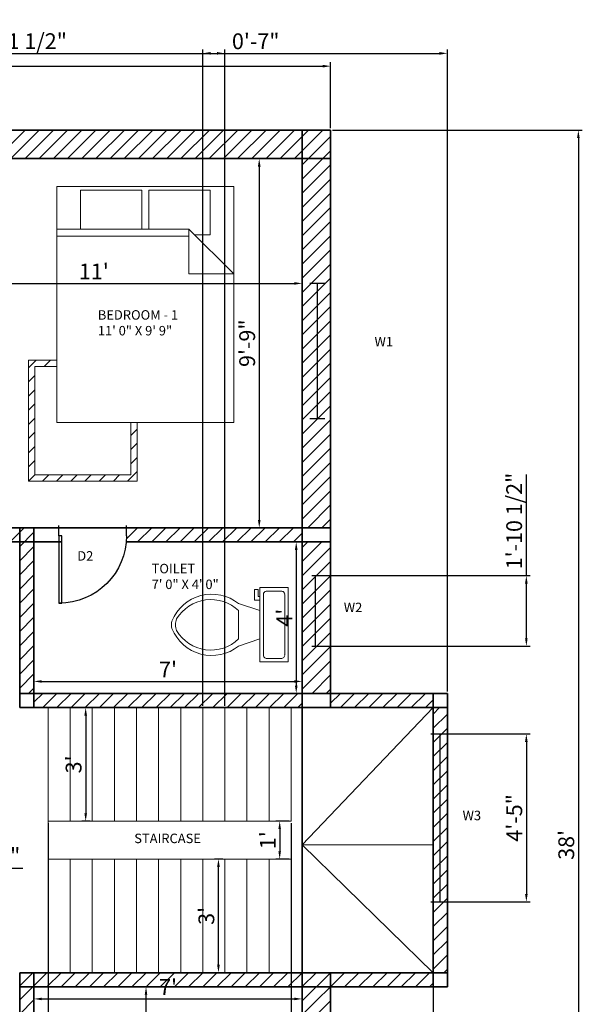
# Model space of a CAD drawing. Units: millimetres. Extents: x 2682 to 3042, y 1647 to 2164.
# Tile 4 of 4: x 2864 to 3042, y 1852 to 2164. Entities that reach past the tile are written whole.
import ezdxf

# ---------------------------------------------------------------- set-up
doc = ezdxf.new("R2010")
doc.units = ezdxf.units.MM
for name, color, linetype, lineweight in [('A-ANNO-TEXT', 170, 'Continuous', 18), ('A-AREA-IDEN', 170, 'Continuous', 18), ('A-FLOR-FIXT', 220, 'Continuous', 18), ('A-WALL-PATT', 3, 'Continuous', 13), ('dimensions', 140, 'Continuous', 18), ('doors', 40, 'Continuous', 25), ('furniture', 220, 'Continuous', 18), ('staircase', 10, 'Continuous', 18), ('walls', 70, 'Continuous', 35), ('windows', 50, 'Continuous', 25)]:
    doc.layers.add(name, color=color, linetype=linetype, lineweight=lineweight)
doc.layers.add('A-FURN-PATT', color=251, linetype='Continuous', lineweight=13, true_color=0x636466)
doc.styles.get("Standard").update_dxf_attribs({"font": 'arial.ttf'})
doc.dimstyles.new('ISO-25', dxfattribs={"dimtxt": 5, "dimasz": 2.5, "dimexe": 1.25, "dimexo": 0.625, "dimtad": 1, "dimdec": 0, "dimlunit": 3, "dimtxsty": 'Standard', "dimcen": 2.5, "dimadec": 0, "dimazin": 0, "dimtfac": 1, "dimtdec": 0, "dimtmove": 0, "dimatfit": 3, "dimfxl": 1, "dimarcsym": 0})

# ---------------------------------------------------------------- blocks, each defined once
blk = doc.blocks.new('*U2')
for p, q in [((0, 0), (0, -6)), ((40, 0), (40, -6))]:
    blk.add_line(p, q)
blk.add_lwpolyline([(0, 0), (0, 40), (1.75, 40), (1.75, 0)], close=True)
blk.add_arc((0, 0), 40, 0, 90)
blk = doc.blocks.new('*U4')
for p, q in [((0, 4), (0, 0)), ((36, 4), (36, 0)), ((0, 2), (36, 2))]:
    blk.add_line(p, q)
blk = doc.blocks.new('*U5')
for p, q in [((0, 4), (0, 0)), ((0, 2), (36, 2)), ((36, 4), (36, 0))]:
    blk.add_line(p, q)
blk = doc.blocks.new('*U6')
for p, q in [((0, 4), (0, 0)), ((36, 4), (36, 0)), ((0, 2), (36, 2))]:
    blk.add_line(p, q)
blk = doc.blocks.new('Toilet - top')
for p, q in [((9.5, -6), (9.5, -2)), ((-8, -8.5), (-8, -8)), ((-7, -8), (-7, -9.5)), ((-4, -8), (-6, -14)), ((4, -8), (6, -14)), ((-10, -8.5), (-8, -8.5)), ((-10, -9.5), (-10, -8.5)), ((-7, -9.5), (-10, -9.5)), ((4, -14), (-4, -14))]:
    blk.add_line(p, q)
blk.add_lwpolyline([(10.5, -8), (10.5, 0), (-10.5, 0), (-10.5, -8)], close=True)
for points in [[(-9.5, -2), (-9.5, -6)], [(8.5, -1), (-8.5, -1)], [(-8.5, -7), (8.5, -7)]]:
    blk.add_lwpolyline(points)
for centre, radius, start, end in [((-8.62, -1.88), 0.884, 81.8699, 188.1301), ((8.62, -1.88), 0.884, 351.8699, 98.1301), ((-8.62, -6.12), 0.884, 171.8699, 278.1301), ((8.62, -6.12), 0.884, 261.8699, 8.1301), ((3.52, -21.58), 12.17, 141.4691, 247.9714), ((4.2, -21.82), 11.33, 136.3677, 238.9468), ((-3.52, -21.58), 12.17, 292.0284, 38.5307), ((-4.2, -21.82), 11.33, 301.053, 43.6321), ((0, -27.88), 4, 245.7318, 294.2682), ((0, -29), 4, 254.8605, 285.1395)]:
    blk.add_arc(centre, radius, start, end)
blk = doc.blocks.new('Bed - Queen')
for p, q in [((0, -80.00003), (0, 0)), ((0, 0), (59.99999, 0)), ((59.99999, 0), (59.99999, -80.00003)), ((7.99999, -1.2), (28.79998, -1.2)), ((7.99999, -14.4), (7.99999, -1.2)), ((28.79998, -1.2), (28.79998, -14.4)), ((31.19999, -1.2), (51.99999, -1.2)), ((31.19999, -14.4), (31.19999, -1.2)), ((51.99999, -1.2), (51.99999, -16.4)), ((0, -14.4), (44.8, -14.4)), ((59.99999, -29.6), (44.8, -14.4)), ((44.8, -14.4), (44.8, -29.6)), ((51.99999, -16.4), (46.79936, -16.4)), ((44.8, -16.8), (0, -16.8)), ((44.8, -29.6), (59.99999, -29.6)), ((59.99999, -80.00003), (0, -80.00003))]:
    blk.add_line(p, q)
blk = doc.blocks.new('*D12')
at = {"layer": 'Defpoints', "color": 0, "transparency": 16777216}
for p in [(2821.09, 2090.07), (2953.09, 2090.07), (2953.09, 2080.38)]:
    blk.add_point(p, dxfattribs=at)
at = {"layer": 'dimensions', "color": 0, "lineweight": -2, "transparency": 16777216}
for p, q in [((2821.09, 2089.45), (2821.09, 2079.13)), ((2953.09, 2089.45), (2953.09, 2079.13)), ((2823.59, 2080.38), (2950.59, 2080.38))]:
    blk.add_line(p, q, dxfattribs=at)
at = {"layer": 'dimensions', "color": 0, "transparency": 16777216}
for points in [[(2823.59, 2080.8), (2823.59, 2079.97), (2821.09, 2080.38)], [(2950.59, 2080.8), (2950.59, 2079.97), (2953.09, 2080.38)]]:
    blk.add_solid(points, dxfattribs=at)
at = {"layer": 'dimensions', "color": 0, "transparency": 16777216, "insert": (2887.09, 2083.52), "char_height": 5, "attachment_point": 5}
blk.add_mtext("11'", dxfattribs=at)
blk = doc.blocks.new('*D13')
at = {"layer": 'Defpoints', "color": 0, "transparency": 16777216}
for p in [(2944.15, 2119.93), (2939.48, 2002.93), (2944.15, 2002.93)]:
    blk.add_point(p, dxfattribs=at)
at = {"layer": 'dimensions', "color": 0, "lineweight": -2, "transparency": 16777216}
for p, q in [((2943.52, 2119.93), (2938.23, 2119.93)), ((2939.48, 2117.43), (2939.48, 2005.43)), ((2943.52, 2002.93), (2938.23, 2002.93))]:
    blk.add_line(p, q, dxfattribs=at)
at = {"layer": 'dimensions', "color": 0, "transparency": 16777216}
for points in [[(2939.07, 2117.43), (2939.9, 2117.43), (2939.48, 2119.93)], [(2939.07, 2005.43), (2939.9, 2005.43), (2939.48, 2002.93)]]:
    blk.add_solid(points, dxfattribs=at)
at = {"layer": 'dimensions', "color": 0, "transparency": 16777216, "insert": (2936.3, 2061.43), "char_height": 5, "attachment_point": 5, "rotation": 90}
blk.add_mtext('9\'-9"', dxfattribs=at)
blk = doc.blocks.new('*D14')
at = {"layer": 'Defpoints', "color": 0, "transparency": 16777216}
for p in [(2868.09, 1954.24), (2953.09, 1954.24), (2953.09, 1954.24)]:
    blk.add_point(p, dxfattribs=at)
at = {"layer": 'dimensions', "color": 0, "lineweight": -2, "transparency": 16777216}
for p, q in [((2868.09, 1954.86), (2868.09, 1955.49)), ((2870.59, 1954.24), (2950.59, 1954.24)), ((2953.09, 1954.86), (2953.09, 1955.49))]:
    blk.add_line(p, q, dxfattribs=at)
at = {"layer": 'dimensions', "color": 0, "transparency": 16777216}
for points in [[(2870.59, 1954.65), (2870.59, 1953.82), (2868.09, 1954.24)], [(2950.59, 1954.65), (2950.59, 1953.82), (2953.09, 1954.24)]]:
    blk.add_solid(points, dxfattribs=at)
at = {"layer": 'dimensions', "color": 0, "transparency": 16777216, "insert": (2910.59, 1957.36), "char_height": 5, "attachment_point": 5}
blk.add_mtext("7' ", dxfattribs=at)
blk = doc.blocks.new('*D15')
at = {"layer": 'Defpoints', "color": 0, "transparency": 16777216}
for p in [(2951.76, 1998.43), (2951.2, 1950.43), (2951.76, 1950.43)]:
    blk.add_point(p, dxfattribs=at)
at = {"layer": 'dimensions', "color": 0, "lineweight": -2, "transparency": 16777216}
for p, q in [((2951.14, 1998.43), (2949.95, 1998.43)), ((2951.2, 1995.93), (2951.2, 1952.93)), ((2951.14, 1950.43), (2949.95, 1950.43))]:
    blk.add_line(p, q, dxfattribs=at)
at = {"layer": 'dimensions', "color": 0, "transparency": 16777216}
for points in [[(2950.79, 1995.93), (2951.62, 1995.93), (2951.2, 1998.43)], [(2950.79, 1952.93), (2951.62, 1952.93), (2951.2, 1950.43)]]:
    blk.add_solid(points, dxfattribs=at)
at = {"layer": 'dimensions', "color": 0, "transparency": 16777216, "insert": (2948.08, 1974.43), "char_height": 5, "attachment_point": 5, "rotation": 90}
blk.add_mtext("4'", dxfattribs=at)
blk = doc.blocks.new('*D16')
at = {"layer": 'Defpoints', "color": 0, "transparency": 16777216}
for p in [(2886.59, 1945.93), (2884.49, 1909.93), (2886.59, 1909.93)]:
    blk.add_point(p, dxfattribs=at)
at = {"layer": 'dimensions', "color": 0, "lineweight": -2, "transparency": 16777216}
for p, q in [((2885.96, 1945.93), (2883.24, 1945.93)), ((2884.49, 1943.43), (2884.49, 1912.43)), ((2885.96, 1909.93), (2883.24, 1909.93))]:
    blk.add_line(p, q, dxfattribs=at)
at = {"layer": 'dimensions', "color": 0, "transparency": 16777216}
for points in [[(2884.08, 1943.43), (2884.91, 1943.43), (2884.49, 1945.93)], [(2884.08, 1912.43), (2884.91, 1912.43), (2884.49, 1909.93)]]:
    blk.add_solid(points, dxfattribs=at)
at = {"layer": 'dimensions', "color": 0, "transparency": 16777216, "insert": (2881.31, 1927.93), "char_height": 5, "attachment_point": 5, "rotation": 90}
blk.add_mtext("3'", dxfattribs=at)
blk = doc.blocks.new('*D17')
at = {"layer": 'Defpoints', "color": 0, "transparency": 16777216}
for p in [(2949.59, 1909.93), (2945.96, 1897.93), (2949.59, 1897.93)]:
    blk.add_point(p, dxfattribs=at)
at = {"layer": 'dimensions', "color": 0, "lineweight": -2, "transparency": 16777216}
for p, q in [((2948.96, 1909.93), (2944.71, 1909.93)), ((2945.96, 1907.43), (2945.96, 1900.43)), ((2948.96, 1897.93), (2944.71, 1897.93))]:
    blk.add_line(p, q, dxfattribs=at)
at = {"layer": 'dimensions', "color": 0, "transparency": 16777216}
for points in [[(2945.54, 1907.43), (2946.37, 1907.43), (2945.96, 1909.93)], [(2945.54, 1900.43), (2946.37, 1900.43), (2945.96, 1897.93)]]:
    blk.add_solid(points, dxfattribs=at)
at = {"layer": 'dimensions', "color": 0, "transparency": 16777216, "insert": (2942.82, 1903.93), "char_height": 5, "attachment_point": 5, "rotation": 90}
blk.add_mtext("1'", dxfattribs=at)
blk = doc.blocks.new('*D18')
at = {"layer": 'Defpoints', "color": 0, "transparency": 16777216}
for p in [(2926.56, 1897.93), (2928.59, 1897.93), (2928.59, 1861.93)]:
    blk.add_point(p, dxfattribs=at)
at = {"layer": 'dimensions', "color": 0, "lineweight": -2, "transparency": 16777216}
for p, q in [((2927.96, 1897.93), (2925.31, 1897.93)), ((2926.56, 1864.43), (2926.56, 1895.43)), ((2927.96, 1861.93), (2925.31, 1861.93))]:
    blk.add_line(p, q, dxfattribs=at)
at = {"layer": 'dimensions', "color": 0, "transparency": 16777216}
for points in [[(2926.14, 1895.43), (2926.98, 1895.43), (2926.56, 1897.93)], [(2926.14, 1864.43), (2926.98, 1864.43), (2926.56, 1861.93)]]:
    blk.add_solid(points, dxfattribs=at)
at = {"layer": 'dimensions', "color": 0, "transparency": 16777216, "insert": (2923.38, 1879.93), "char_height": 5, "attachment_point": 5, "rotation": 90}
blk.add_mtext("3'", dxfattribs=at)
blk = doc.blocks.new('*D19')
at = {"layer": 'Defpoints', "color": 0, "transparency": 16777216}
for p in [(2868.09, 1853.61), (2953.09, 1853.61), (2953.09, 1853.61)]:
    blk.add_point(p, dxfattribs=at)
at = {"layer": 'dimensions', "color": 0, "lineweight": -2, "transparency": 16777216}
for p, q in [((2868.09, 1854.23), (2868.09, 1854.86)), ((2953.09, 1854.23), (2953.09, 1854.86)), ((2870.59, 1853.61), (2950.59, 1853.61))]:
    blk.add_line(p, q, dxfattribs=at)
at = {"layer": 'dimensions', "color": 0, "transparency": 16777216}
for points in [[(2870.59, 1854.02), (2870.59, 1853.19), (2868.09, 1853.61)], [(2950.59, 1854.02), (2950.59, 1853.19), (2953.09, 1853.61)]]:
    blk.add_solid(points, dxfattribs=at)
at = {"layer": 'dimensions', "color": 0, "transparency": 16777216, "insert": (2910.59, 1856.73), "char_height": 5, "attachment_point": 5}
blk.add_mtext("7'", dxfattribs=at)
blk = doc.blocks.new('*D20')
at = {"layer": 'Defpoints', "color": 0, "transparency": 16777216}
for p in [(2903.61, 1857.43), (2911.95, 1857.43), (2911.95, 1809.43)]:
    blk.add_point(p, dxfattribs=at)
at = {"layer": 'dimensions', "color": 0, "lineweight": -2, "transparency": 16777216}
for p, q in [((2911.33, 1857.43), (2902.36, 1857.43)), ((2903.61, 1811.93), (2903.61, 1854.93)), ((2911.33, 1809.43), (2902.36, 1809.43))]:
    blk.add_line(p, q, dxfattribs=at)
at = {"layer": 'dimensions', "color": 0, "transparency": 16777216}
for points in [[(2903.19, 1854.93), (2904.02, 1854.93), (2903.61, 1857.43)], [(2903.19, 1811.93), (2904.02, 1811.93), (2903.61, 1809.43)]]:
    blk.add_solid(points, dxfattribs=at)
at = {"layer": 'dimensions', "color": 0, "transparency": 16777216, "insert": (2900.48, 1833.43), "char_height": 5, "attachment_point": 5, "rotation": 90}
blk.add_mtext("4'", dxfattribs=at)
blk = doc.blocks.new('*D27')
at = {"layer": 'Defpoints', "color": 0, "transparency": 16777216}
for p in [(2962.09, 2128.93), (2962.09, 1675.93), (3040.59, 1675.93)]:
    blk.add_point(p, dxfattribs=at)
at = {"layer": 'dimensions', "color": 0, "lineweight": -2, "transparency": 16777216}
for p, q in [((2962.71, 2128.93), (3041.84, 2128.93)), ((3040.59, 2126.43), (3040.59, 1678.43)), ((2962.71, 1675.93), (3041.84, 1675.93))]:
    blk.add_line(p, q, dxfattribs=at)
at = {"layer": 'dimensions', "color": 0, "transparency": 16777216}
for points in [[(3040.17, 2126.43), (3041, 2126.43), (3040.59, 2128.93)], [(3040.17, 1678.43), (3041, 1678.43), (3040.59, 1675.93)]]:
    blk.add_solid(points, dxfattribs=at)
at = {"layer": 'dimensions', "color": 0, "transparency": 16777216, "insert": (3037.41, 1902.43), "char_height": 5, "attachment_point": 5, "rotation": 90}
blk.add_mtext("38'", dxfattribs=at)
blk = doc.blocks.new('*D28')
at = {"layer": 'Defpoints', "color": 0, "transparency": 16777216}
for p in [(2962.09, 2149.24), (2723.59, 2128.93), (2962.09, 2128.93)]:
    blk.add_point(p, dxfattribs=at)
at = {"layer": 'dimensions', "color": 0, "lineweight": -2, "transparency": 16777216}
for p, q in [((2723.59, 2129.55), (2723.59, 2150.49)), ((2962.09, 2129.55), (2962.09, 2150.49)), ((2726.09, 2149.24), (2959.59, 2149.24))]:
    blk.add_line(p, q, dxfattribs=at)
at = {"layer": 'dimensions', "color": 0, "transparency": 16777216}
for points in [[(2726.09, 2149.66), (2726.09, 2148.82), (2723.59, 2149.24)], [(2959.59, 2149.66), (2959.59, 2148.82), (2962.09, 2149.24)]]:
    blk.add_solid(points, dxfattribs=at)
at = {"layer": 'dimensions', "color": 0, "transparency": 16777216, "insert": (2842.84, 2152.42), "char_height": 5, "width": 20.59, "attachment_point": 5}
blk.add_mtext("20'", dxfattribs=at)
blk = doc.blocks.new('*D49')
at = {"layer": 'Defpoints', "color": 0, "transparency": 16777216}
for p in [(2772.38, 1900.42), (2807.82, 1900.42), (2807.82, 1895.1)]:
    blk.add_point(p, dxfattribs=at)
at = {"layer": 'dimensions', "color": 0, "lineweight": -2, "transparency": 16777216}
for p, q in [((2772.38, 1899.79), (2772.38, 1893.85)), ((2807.82, 1899.79), (2807.82, 1893.85)), ((2774.88, 1895.1), (2805.32, 1895.1)), ((2807.82, 1895.1), (2864.59, 1895.1))]:
    blk.add_line(p, q, dxfattribs=at)
at = {"layer": 'dimensions', "color": 0, "transparency": 16777216}
for points in [[(2774.88, 1895.52), (2774.88, 1894.69), (2772.38, 1895.1)], [(2805.32, 1895.52), (2805.32, 1894.69), (2807.82, 1895.1)]]:
    blk.add_solid(points, dxfattribs=at)
at = {"layer": 'dimensions', "color": 0, "transparency": 16777216, "insert": (2837.46, 1898.31), "char_height": 5, "attachment_point": 5}
blk.add_mtext('TABLE 2\'-11 1/2"', dxfattribs=at)
blk = doc.blocks.new('*D53')
at = {"layer": 'Defpoints', "color": 0, "transparency": 16777216}
for p in [(2999.09, 2153.3), (2723.59, 2128.93), (2999.09, 1950.43)]:
    blk.add_point(p, dxfattribs=at)
at = {"layer": 'dimensions', "color": 0, "lineweight": -2, "transparency": 16777216}
for p, q in [((2723.59, 2129.55), (2723.59, 2154.55)), ((2726.09, 2153.3), (2996.59, 2153.3)), ((2999.09, 1951.05), (2999.09, 2154.55))]:
    blk.add_line(p, q, dxfattribs=at)
at = {"layer": 'dimensions', "color": 0, "transparency": 16777216}
for points in [[(2726.09, 2153.72), (2726.09, 2152.88), (2723.59, 2153.3)], [(2996.59, 2153.72), (2996.59, 2152.88), (2999.09, 2153.3)]]:
    blk.add_solid(points, dxfattribs=at)
at = {"layer": 'dimensions', "color": 0, "transparency": 16777216, "insert": (2861.34, 2156.51), "char_height": 5, "attachment_point": 5}
blk.add_mtext('22\'-11 1/2"', dxfattribs=at)
blk = doc.blocks.new('*D54')
at = {"layer": 'Defpoints', "color": 0, "transparency": 16777216}
for p in [(2872.59, 1909.93), (2949.59, 1909.93), (2949.59, 1651.55)]:
    blk.add_point(p, dxfattribs=at)
at = {"layer": 'dimensions', "color": 0, "lineweight": -2, "transparency": 16777216}
for p, q in [((2872.59, 1909.3), (2872.59, 1650.3)), ((2949.59, 1909.3), (2949.59, 1650.3)), ((2875.09, 1651.55), (2947.09, 1651.55))]:
    blk.add_line(p, q, dxfattribs=at)
at = {"layer": 'dimensions', "color": 0, "transparency": 16777216}
for points in [[(2875.09, 1651.97), (2875.09, 1651.13), (2872.59, 1651.55)], [(2947.09, 1651.97), (2947.09, 1651.13), (2949.59, 1651.55)]]:
    blk.add_solid(points, dxfattribs=at)
at = {"layer": 'dimensions', "color": 0, "transparency": 16777216, "insert": (2911.09, 1654.73), "char_height": 5, "attachment_point": 5}
blk.add_mtext('6\'-5"', dxfattribs=at)
blk = doc.blocks.new('*D55')
at = {"layer": 'Defpoints', "color": 0, "transparency": 16777216}
for p in [(2953.09, 1902.43), (2994.59, 1861.93), (2994.59, 1651.55)]:
    blk.add_point(p, dxfattribs=at)
at = {"layer": 'dimensions', "color": 0, "lineweight": -2, "transparency": 16777216}
for p, q in [((2953.09, 1901.8), (2953.09, 1650.3)), ((2994.59, 1861.3), (2994.59, 1650.3)), ((2955.59, 1651.55), (2992.09, 1651.55))]:
    blk.add_line(p, q, dxfattribs=at)
at = {"layer": 'dimensions', "color": 0, "transparency": 16777216}
for points in [[(2955.59, 1651.97), (2955.59, 1651.13), (2953.09, 1651.55)], [(2992.09, 1651.97), (2992.09, 1651.13), (2994.59, 1651.55)]]:
    blk.add_solid(points, dxfattribs=at)
at = {"layer": 'dimensions', "color": 0, "transparency": 16777216, "insert": (2973.84, 1654.76), "char_height": 5, "attachment_point": 5}
blk.add_mtext('3\'-5 1/2"', dxfattribs=at)
blk = doc.blocks.new('*D57')
at = {"layer": 'Defpoints', "color": 0, "transparency": 16777216}
for p in [(2957.36, 1987.76), (3024.11, 1987.76), (2957.36, 1965.41)]:
    blk.add_point(p, dxfattribs=at)
at = {"layer": 'dimensions', "color": 0, "lineweight": -2, "transparency": 16777216}
for p, q in [((3024.11, 1987.76), (3024.11, 2019.87)), ((2957.98, 1987.76), (3025.36, 1987.76)), ((3024.11, 1967.91), (3024.11, 1985.26)), ((2957.98, 1965.41), (3025.36, 1965.41))]:
    blk.add_line(p, q, dxfattribs=at)
at = {"layer": 'dimensions', "color": 0, "transparency": 16777216}
for points in [[(3023.69, 1985.26), (3024.52, 1985.26), (3024.11, 1987.76)], [(3023.69, 1967.91), (3024.52, 1967.91), (3024.11, 1965.41)]]:
    blk.add_solid(points, dxfattribs=at)
at = {"layer": 'dimensions', "color": 0, "transparency": 16777216, "insert": (3020.89, 2005.07), "char_height": 5, "attachment_point": 5, "rotation": 90}
blk.add_mtext('1\'-10 1/2"', dxfattribs=at)
blk = doc.blocks.new('*D58')
at = {"layer": 'Defpoints', "color": 0, "transparency": 16777216}
for p in [(2996.77, 1937.59), (2996.77, 1884.37), (3024.11, 1884.37)]:
    blk.add_point(p, dxfattribs=at)
at = {"layer": 'dimensions', "color": 0, "lineweight": -2, "transparency": 16777216}
for p, q in [((2997.4, 1937.59), (3025.36, 1937.59)), ((3024.11, 1935.09), (3024.11, 1886.87)), ((2997.4, 1884.37), (3025.36, 1884.37))]:
    blk.add_line(p, q, dxfattribs=at)
at = {"layer": 'dimensions', "color": 0, "transparency": 16777216}
for points in [[(3023.69, 1935.09), (3024.52, 1935.09), (3024.11, 1937.59)], [(3023.69, 1886.87), (3024.52, 1886.87), (3024.11, 1884.37)]]:
    blk.add_solid(points, dxfattribs=at)
at = {"layer": 'dimensions', "color": 0, "transparency": 16777216, "insert": (3020.94, 1910.98), "char_height": 5, "attachment_point": 5, "rotation": 90}
blk.add_mtext('4\'-5"', dxfattribs=at)
blk = doc.blocks.new('*D65')
at = {"layer": 'Defpoints', "color": 0, "transparency": 16777216}
for p in [(2928.59, 2153.3), (2921.59, 1945.93), (2928.59, 1945.93)]:
    blk.add_point(p, dxfattribs=at)
at = {"layer": 'dimensions', "color": 0, "lineweight": -2, "transparency": 16777216}
for p, q in [((2921.59, 1946.55), (2921.59, 2154.55)), ((2924.09, 2153.3), (2926.09, 2153.3)), ((2928.59, 1946.55), (2928.59, 2154.55)), ((2928.59, 2153.3), (2945.63, 2153.3))]:
    blk.add_line(p, q, dxfattribs=at)
at = {"layer": 'dimensions', "color": 0, "transparency": 16777216}
for points in [[(2924.09, 2153.72), (2924.09, 2152.88), (2921.59, 2153.3)], [(2926.09, 2153.72), (2926.09, 2152.88), (2928.59, 2153.3)]]:
    blk.add_solid(points, dxfattribs=at)
at = {"layer": 'dimensions', "color": 0, "transparency": 16777216, "insert": (2938.36, 2156.48), "char_height": 5, "attachment_point": 5}
blk.add_mtext('0\'-7"', dxfattribs=at)

msp = doc.modelspace()

# ---------------------------------------------------------------- hatches: boundary and pattern name
at = {"layer": 'A-FURN-PATT'}
h = msp.add_hatch(dxfattribs=at)
h.set_pattern_fill('ANSI31', color=256)
h.paths.add_polyline_path([(2868.36, 2054.1), (2875.35, 2054.1), (2875.35, 2056.1), (2866.36, 2056.1), (2866.36, 2017.68), (2900.8, 2017.68), (2900.8, 2036.29), (2898.8, 2036.29), (2898.8, 2019.68), (2868.36, 2019.68)])
h.paths.add_polyline_path([(2907.02, 1780.81), (2865.81, 1780.81), (2865.81, 1749.67), (2875.45, 1749.67), (2875.45, 1751.67), (2867.81, 1751.67), (2867.81, 1778.81), (2905.02, 1778.81), (2905.02, 1774.7), (2907.02, 1774.7)])
at = {"layer": 'A-WALL-PATT'}
h = msp.add_hatch(dxfattribs=at)
h.set_pattern_fill('ANSI31', color=256)
h.paths.add_polyline_path([(2816.59, 2128.93), (2732.59, 2128.93), (2732.59, 2119.93), (2816.59, 2119.93)])
h.paths.add_polyline_path([(2953.09, 2128.93), (2821.09, 2128.93), (2821.09, 2119.93), (2953.09, 2119.93)])
h.paths.add_polyline_path([(2821.09, 2119.93), (2816.59, 2119.93), (2816.59, 2002.93), (2821.09, 2002.93)])
h.paths.add_polyline_path([(2821.09, 2128.93), (2816.59, 2128.93), (2816.59, 2119.93), (2821.09, 2119.93)])
h.paths.add_polyline_path([(2732.59, 2119.93), (2723.59, 2119.93), (2723.59, 2002.93), (2732.59, 2002.93)])
h.paths.add_polyline_path([(2732.59, 2128.93), (2723.59, 2128.93), (2723.59, 2119.93), (2732.59, 2119.93)])
h.paths.add_polyline_path([(2962.09, 2119.93), (2953.09, 2119.93), (2953.09, 2002.93), (2962.09, 2002.93)])
h.paths.add_polyline_path([(2962.09, 2128.93), (2953.09, 2128.93), (2953.09, 2119.93), (2962.09, 2119.93)])
h.paths.add_polyline_path([(2953.09, 2002.93), (2897.45, 2002.93), (2897.45, 2000.43, -0.023466), (2897.35, 1998.43), (2953.09, 1998.43)])
h.paths.add_polyline_path([(2962.09, 1998.43), (2953.09, 1998.43), (2953.09, 1950.43), (2962.09, 1950.43)])
h.paths.add_polyline_path([(2953.09, 1950.43), (2868.09, 1950.43), (2868.09, 1945.93), (2953.09, 1945.93)])
h.paths.add_polyline_path([(2994.59, 1950.43), (2962.09, 1950.43), (2962.09, 1945.93), (2994.59, 1945.93)])
h.paths.add_polyline_path([(2868.09, 1998.43), (2863.59, 1998.43), (2863.59, 1950.43), (2868.09, 1950.43)])
h.paths.add_polyline_path([(2868.09, 2002.93), (2863.59, 2002.93), (2863.59, 1998.43), (2868.09, 1998.43)])
h.paths.add_polyline_path([(2863.59, 2002.93), (2853.46, 2002.93, -0.011786), (2853.49, 2001.52), (2853.49, 1998.43), (2863.59, 1998.43)])
h.paths.add_polyline_path([(2783.8, 2001.45, -0.012351), (2783.84, 2002.93), (2756.59, 2002.93), (2756.59, 2002.69), (2732.59, 2002.93), (2732.59, 1998.43), (2783.8, 1998.43)])
h.paths.add_polyline_path([(2732.59, 2002.93), (2723.59, 2002.93), (2723.59, 1998.43), (2732.59, 1998.43)])
h.paths.add_polyline_path([(2732.59, 1998.43), (2723.59, 1998.43), (2723.59, 1809.43), (2732.59, 1809.43)])
h.paths.add_polyline_path([(2994.59, 1861.93), (2962.09, 1861.93), (2962.09, 1857.43), (2994.59, 1857.43)])
h.paths.add_polyline_path([(2999.09, 1884.37), (2994.59, 1884.37), (2994.59, 1861.93), (2999.09, 1861.93)])
h.paths.add_polyline_path([(2953.09, 1861.93), (2868.09, 1861.93), (2868.09, 1857.43), (2953.09, 1857.43)])
h.paths.add_polyline_path([(2962.09, 1861.93), (2953.09, 1861.93), (2953.09, 1857.43), (2962.09, 1857.43)])
h.paths.add_polyline_path([(2868.09, 1857.43), (2863.59, 1857.43), (2863.59, 1831.73), (2866.39, 1831.73, -0.019816), (2868.09, 1831.66)])
h.paths.add_polyline_path([(2868.09, 1861.93), (2863.59, 1861.93), (2863.59, 1857.43), (2868.09, 1857.43)])
h.paths.add_polyline_path([(2962.09, 1804.93), (2953.09, 1804.93), (2953.09, 1684.93), (2962.09, 1684.93)])
h.paths.add_polyline_path([(2962.09, 1857.43), (2953.09, 1857.43), (2953.09, 1809.43), (2962.09, 1809.43)])
h.paths.add_polyline_path([(2962.09, 1809.43), (2953.09, 1809.43), (2953.09, 1804.93), (2962.09, 1804.93)])
h.paths.add_polyline_path([(2953.09, 1809.43), (2868.09, 1809.43), (2868.09, 1804.93), (2953.09, 1804.93)])
h.paths.add_polyline_path([(2868.09, 1809.43), (2863.59, 1809.43), (2863.59, 1804.93), (2868.09, 1804.93)])
h.paths.add_polyline_path([(2863.59, 1809.43), (2855.42, 1809.43), (2855.42, 1805.73, -0.006742), (2855.41, 1804.93), (2863.59, 1804.93)])
h.paths.add_polyline_path([(2953.09, 1684.93), (2863.59, 1684.93), (2821.09, 1684.93), (2821.09, 1675.93), (2863.59, 1675.93), (2953.09, 1675.93)])
h.paths.add_polyline_path([(2962.09, 1684.93), (2953.09, 1684.93), (2953.09, 1675.93), (2962.09, 1675.93)])
h.paths.add_polyline_path([(2821.09, 1804.93), (2816.59, 1804.93), (2816.59, 1704.93), (2821.09, 1704.93)])
h.paths.add_polyline_path([(2821.09, 1695.93), (2816.59, 1695.93), (2816.59, 1684.93), (2821.09, 1684.93)])
h.paths.add_polyline_path([(2821.09, 1704.93), (2816.59, 1704.93), (2816.59, 1695.93), (2821.09, 1695.93)])
h.paths.add_polyline_path([(2821.09, 1684.93), (2816.59, 1684.93), (2816.59, 1675.93), (2821.09, 1675.93)])
h.paths.add_polyline_path([(2776.38, 1700.56, -0.030957), (2776.65, 1704.93), (2732.59, 1704.93), (2732.59, 1695.93), (2776.38, 1695.93)])
h.paths.add_polyline_path([(2732.59, 1804.93), (2723.59, 1804.93), (2723.59, 1704.93), (2732.59, 1704.93)])
h.paths.add_polyline_path([(2732.59, 1704.93), (2723.59, 1704.93), (2723.59, 1695.93), (2732.59, 1695.93)])
h.paths.add_polyline_path([(2999.09, 1945.93), (2994.59, 1945.93), (2994.59, 1937.59), (2999.09, 1937.59)])
h.paths.add_polyline_path([(2999.09, 1937.59), (2996.77, 1937.59), (2996.77, 1884.37), (2999.09, 1884.37)])
h.paths.add_polyline_path([(2996.77, 1937.59), (2994.59, 1937.59), (2994.59, 1884.37), (2996.77, 1884.37)])
h.paths.add_polyline_path([(2784.83, 1809.43), (2732.59, 1809.43), (2732.59, 1804.93), (2784.84, 1804.93, -0.006742), (2784.83, 1805.73)])
h.paths.add_polyline_path([(2732.59, 1809.43), (2723.59, 1809.43), (2723.59, 1804.93), (2732.59, 1804.93)])

# ---------------------------------------------------------------- linework, layer by layer
at = {"layer": 'furniture'}
for p, q in [((2875.35, 2056.1), (2866.36, 2056.1)), ((2866.36, 2056.1), (2866.36, 2017.68)), ((2875.35, 2054.1), (2868.36, 2054.1)), ((2868.36, 2054.1), (2868.36, 2019.68)), ((2898.8, 2019.68), (2898.8, 2036.29)), ((2900.8, 2017.68), (2900.8, 2036.29)), ((2868.36, 2019.68), (2898.8, 2019.68)), ((2866.36, 2017.68), (2900.8, 2017.68))]:
    msp.add_line(p, q, dxfattribs=at)
at = {"layer": 'staircase'}
for p, q in [((2872.59, 1930.6), (2872.59, 1945.93)), ((2872.59, 1945.93), (2872.59, 1861.93)), ((2879.59, 1945.93), (2879.59, 1909.93)), ((2886.59, 1945.93), (2886.59, 1909.93)), ((2893.59, 1945.93), (2893.59, 1909.93)), ((2900.59, 1945.93), (2900.59, 1909.93)), ((2907.59, 1945.93), (2907.59, 1909.93)), ((2914.59, 1945.93), (2914.59, 1909.93)), ((2921.59, 1945.93), (2921.59, 1909.93)), ((2928.59, 1945.93), (2928.59, 1909.93)), ((2935.59, 1945.93), (2935.59, 1909.93)), ((2942.59, 1945.93), (2942.59, 1909.93)), ((2949.59, 1945.93), (2949.59, 1909.93)), ((2953.09, 1902.43), (2994.59, 1945.93)), ((2879.59, 1909.93), (2872.59, 1909.93)), ((2879.59, 1909.93), (2949.59, 1909.93)), ((2953.09, 1902.43), (2994.59, 1861.93)), ((2953.09, 1902.43), (2994.59, 1902.43)), ((2872.59, 1861.93), (2872.59, 1897.93)), ((2879.59, 1897.93), (2872.59, 1897.93)), ((2879.59, 1861.93), (2879.59, 1897.93)), ((2949.59, 1897.93), (2879.59, 1897.93)), ((2886.59, 1861.93), (2886.59, 1897.93)), ((2893.59, 1861.93), (2893.59, 1897.93)), ((2900.59, 1861.93), (2900.59, 1897.93)), ((2907.59, 1861.93), (2907.59, 1897.93)), ((2914.59, 1861.93), (2914.59, 1897.93)), ((2921.59, 1861.93), (2921.59, 1897.93)), ((2928.59, 1861.93), (2928.59, 1897.93)), ((2935.59, 1861.93), (2935.59, 1897.93)), ((2942.59, 1861.93), (2942.59, 1897.93)), ((2949.59, 1861.93), (2949.59, 1897.93))]:
    msp.add_line(p, q, dxfattribs=at)
at = {"layer": 'walls'}
for p, q in [((2723.59, 2128.93), (2962.09, 2128.93)), ((2953.09, 2128.93), (2953.09, 1675.93)), ((2962.09, 2128.93), (2962.09, 1945.93)), ((2723.59, 2119.93), (2962.09, 2119.93)), ((2853.46, 2002.93), (2962.09, 2002.93)), ((2863.59, 2002.93), (2863.59, 1945.93)), ((2868.09, 2002.93), (2868.09, 1945.93)), ((2723.59, 1998.43), (2876.97, 1998.43)), ((2897.35, 1998.43), (2962.09, 1998.43)), ((2863.59, 1950.43), (2962.09, 1950.43)), ((2962.09, 1950.43), (2999.09, 1950.43)), ((2994.59, 1950.43), (2994.59, 1857.43)), ((2999.09, 1950.43), (2999.09, 1857.43)), ((2863.59, 1945.93), (2962.09, 1945.93)), ((2962.09, 1945.93), (2999.09, 1945.93)), ((2863.59, 1861.93), (2962.09, 1861.93)), ((2863.59, 1861.93), (2863.59, 1804.93)), ((2868.09, 1861.93), (2868.09, 1831.66)), ((2999.09, 1861.93), (2962.09, 1861.93)), ((2962.09, 1861.93), (2962.09, 1675.93)), ((2863.59, 1857.43), (2962.09, 1857.43)), ((2999.09, 1857.43), (2962.09, 1857.43))]:
    msp.add_line(p, q, dxfattribs=at)

# ---------------------------------------------------------------- block references
at = {"layer": 'A-FLOR-FIXT', "xscale": 1.121371250506495, "yscale": 1.121371250506495, "zscale": 1.121371250506495, "rotation": 269.9999999999973}
msp.add_blockref('Toilet - top', (2948.66, 1972.18), dxfattribs=at)
at = {"layer": 'doors', "xscale": -0.5354065160128529, "yscale": 0.5354065160128529, "zscale": 0.5354065160128529, "rotation": 180}
msp.add_blockref('*U2', (2876.03, 2000.43), dxfattribs=at)
at = {"layer": 'furniture', "xscale": 0.9346925861226617, "yscale": 0.9346925861226617, "zscale": 0.9346925861226617}
msp.add_blockref('Bed - Queen', (2875.35, 2111.06), dxfattribs=at)
at = {"layer": 'windows'}
for name, p, xscale, yscale, zscale, rotation in [('*U4', (2955.47, 2080.38), 1.192221816707046, 1.192221816707046, 1.192221816707046, 270), ('*U5', (2958.6, 1965.41), 0.6208711624712905, 0.6208711624712905, 0.6208711624712905, 90), ('*U6', (2999.73, 1884.37), 1.478434873366294, 1.478434873366294, 1.478434873366294, 90)]:
    msp.add_blockref(name, p, dxfattribs=dict(at, xscale=xscale, yscale=yscale, zscale=zscale, rotation=rotation))

# ---------------------------------------------------------------- texts
at = {"layer": 'A-ANNO-TEXT', "char_height": 3, "attachment_point": 1}
for s, width, insert in [('W1', 21.5834, (2976.01, 2063.41)), ('D2', 9.7571, (2881.83, 1995.52)), ('W2', 13.5636, (2966.27, 1979.19)), ('W3', 17.3495, (3003.91, 1913.26))]:
    msp.add_mtext_dynamic_manual_height_columns(s, width=width, gutter_width=12.5, heights=[0], dxfattribs=dict(at, insert=insert))
at = {"layer": 'A-AREA-IDEN', "char_height": 3, "attachment_point": 1}
for s, width, insert in [('BEDROOM - 1 \\P11\' 0" X 9\' 9"', 30.2204, (2888.35, 2071.9)), ('TOILET\\P7\' 0" X 4\' 0"', 36.8029, (2905.39, 1991.51)), ('STAIRCASE', 26.371, (2899.88, 1905.99))]:
    msp.add_mtext_dynamic_manual_height_columns(s, width=width, gutter_width=12.5, heights=[0], dxfattribs=dict(at, insert=insert))

# ---------------------------------------------------------------- dimensions: what is measured, and where the dimension line sits
at = {"layer": 'dimensions'}
for base, p1, p2, override, picture, middle in [((2999.09, 2153.3), (2723.59, 2128.93), (2999.09, 1950.43), {"dimdec": 1, "dimlfac": 1, "dimrnd": 0, "dimzin": 1, "dimdsep": 46, "dimlunit": 4, "dimfrac": 2}, '*D53', (2861.34, 2156.51)), ((2928.59, 2153.3), (2921.59, 1945.93), (2928.59, 1945.93), {"dimdec": 1, "dimlfac": 1, "dimrnd": 0, "dimzin": 1, "dimdsep": 46, "dimlunit": 4, "dimfrac": 2}, '*D65', (2938.36, 2156.48)), ((2953.09, 2080.38), (2821.09, 2090.07), (2953.09, 2090.07), {"dimclrd": 0, "dimclre": 0, "dimclrt": 0}, '*D12', (2887.09, 2083.52)), ((2949.59, 1651.55), (2872.59, 1909.93), (2949.59, 1909.93), {"dimdec": 1, "dimlfac": 1, "dimrnd": 0, "dimzin": 1, "dimdsep": 46, "dimlunit": 4, "dimfrac": 2}, '*D54', (2911.09, 1654.73)), ((2994.59, 1651.55), (2953.09, 1902.43), (2994.59, 1861.93), {"dimdec": 1, "dimlfac": 1, "dimrnd": 0, "dimzin": 1, "dimdsep": 46, "dimlunit": 4, "dimfrac": 2}, '*D55', (2973.84, 1654.76))]:
    dim = msp.add_linear_dim(base=base, p1=p1, p2=p2, dimstyle='ISO-25', override=override, dxfattribs=at)
    dim.commit()
    dim.dimension.update_dxf_attribs({"geometry": picture, "text_midpoint": middle})
for base, p1, p2, text, override, picture, middle in [((2962.09, 2149.24), (2723.59, 2128.93), (2962.09, 2128.93), "20'", {"dimclrd": 0, "dimclre": 0, "dimclrt": 0}, '*D28', (2842.84, 2152.42)), ((2953.09, 1954.24), (2868.09, 1954.24), (2953.09, 1954.24), "7' ", {"dimclrd": 0, "dimclre": 0, "dimclrt": 0}, '*D14', (2910.59, 1957.36)), ((2807.82, 1895.1), (2772.38, 1900.42), (2807.82, 1900.42), 'TABLE <>', {"dimdec": 1, "dimlfac": 1, "dimrnd": 0, "dimzin": 1, "dimdsep": 46, "dimlunit": 4, "dimfrac": 2}, '*D49', (2837.46, 1898.31)), ((2953.09, 1853.61), (2868.09, 1853.61), (2953.09, 1853.61), "7'", {"dimclrd": 0, "dimclre": 0, "dimclrt": 0}, '*D19', (2910.59, 1856.73))]:
    dim = msp.add_linear_dim(base=base, p1=p1, p2=p2, text=text, dimstyle='ISO-25', override=override, dxfattribs=at)
    dim.commit()
    dim.dimension.update_dxf_attribs({"geometry": picture, "text_midpoint": middle})
dim = msp.add_linear_dim(base=(3040.59, 1675.93), p1=(2962.09, 2128.93), p2=(2962.09, 1675.93), angle=90, text="38'", dimstyle='ISO-25', override={"dimclrd": 0, "dimclre": 0, "dimclrt": 0}, dxfattribs=at)
dim.commit()
dim.dimension.update_dxf_attribs({"geometry": '*D27', "text_midpoint": (3037.41, 1902.43)})
for base, p1, p2, override, picture, middle in [((2939.48, 2002.93), (2944.15, 2119.93), (2944.15, 2002.93), {"dimclrd": 0, "dimclre": 0, "dimclrt": 0}, '*D13', (2936.3, 2061.43)), ((3024.1051, 1987.7638), (2957.3595, 1965.4124), (2957.3595, 1987.7638), {"dimdec": 1, "dimlfac": 1, "dimrnd": 0, "dimzin": 1, "dimdsep": 46, "dimlunit": 4, "dimfrac": 2}, '*D57', (3020.8948, 2005.0668)), ((2951.2, 1950.43), (2951.76, 1998.43), (2951.76, 1950.43), {"dimclrd": 0, "dimclre": 0, "dimclrt": 0}, '*D15', (2948.08, 1974.43)), ((2884.49, 1909.93), (2886.59, 1945.93), (2886.59, 1909.93), {"dimclrd": 0, "dimclre": 0, "dimclrt": 0}, '*D16', (2881.31, 1927.93)), ((3024.11, 1884.37), (2996.77, 1937.59), (2996.77, 1884.37), {"dimdec": 1, "dimlfac": 1, "dimrnd": 0, "dimzin": 1, "dimdsep": 46, "dimlunit": 4, "dimfrac": 2}, '*D58', (3020.94, 1910.98)), ((2945.96, 1897.93), (2949.59, 1909.93), (2949.59, 1897.93), {"dimclrd": 0, "dimclre": 0, "dimclrt": 0}, '*D17', (2942.82, 1903.93)), ((2926.56, 1897.93), (2928.59, 1861.93), (2928.59, 1897.93), {"dimclrd": 0, "dimclre": 0, "dimclrt": 0}, '*D18', (2923.38, 1879.93)), ((2903.61, 1857.43), (2911.95, 1809.43), (2911.95, 1857.43), {"dimclrd": 0, "dimclre": 0, "dimclrt": 0}, '*D20', (2900.48, 1833.43))]:
    dim = msp.add_linear_dim(base=base, p1=p1, p2=p2, angle=90, dimstyle='ISO-25', override=override, dxfattribs=at)
    dim.commit()
    dim.dimension.update_dxf_attribs({"geometry": picture, "text_midpoint": middle})

doc.saveas('drawing.dxf')
